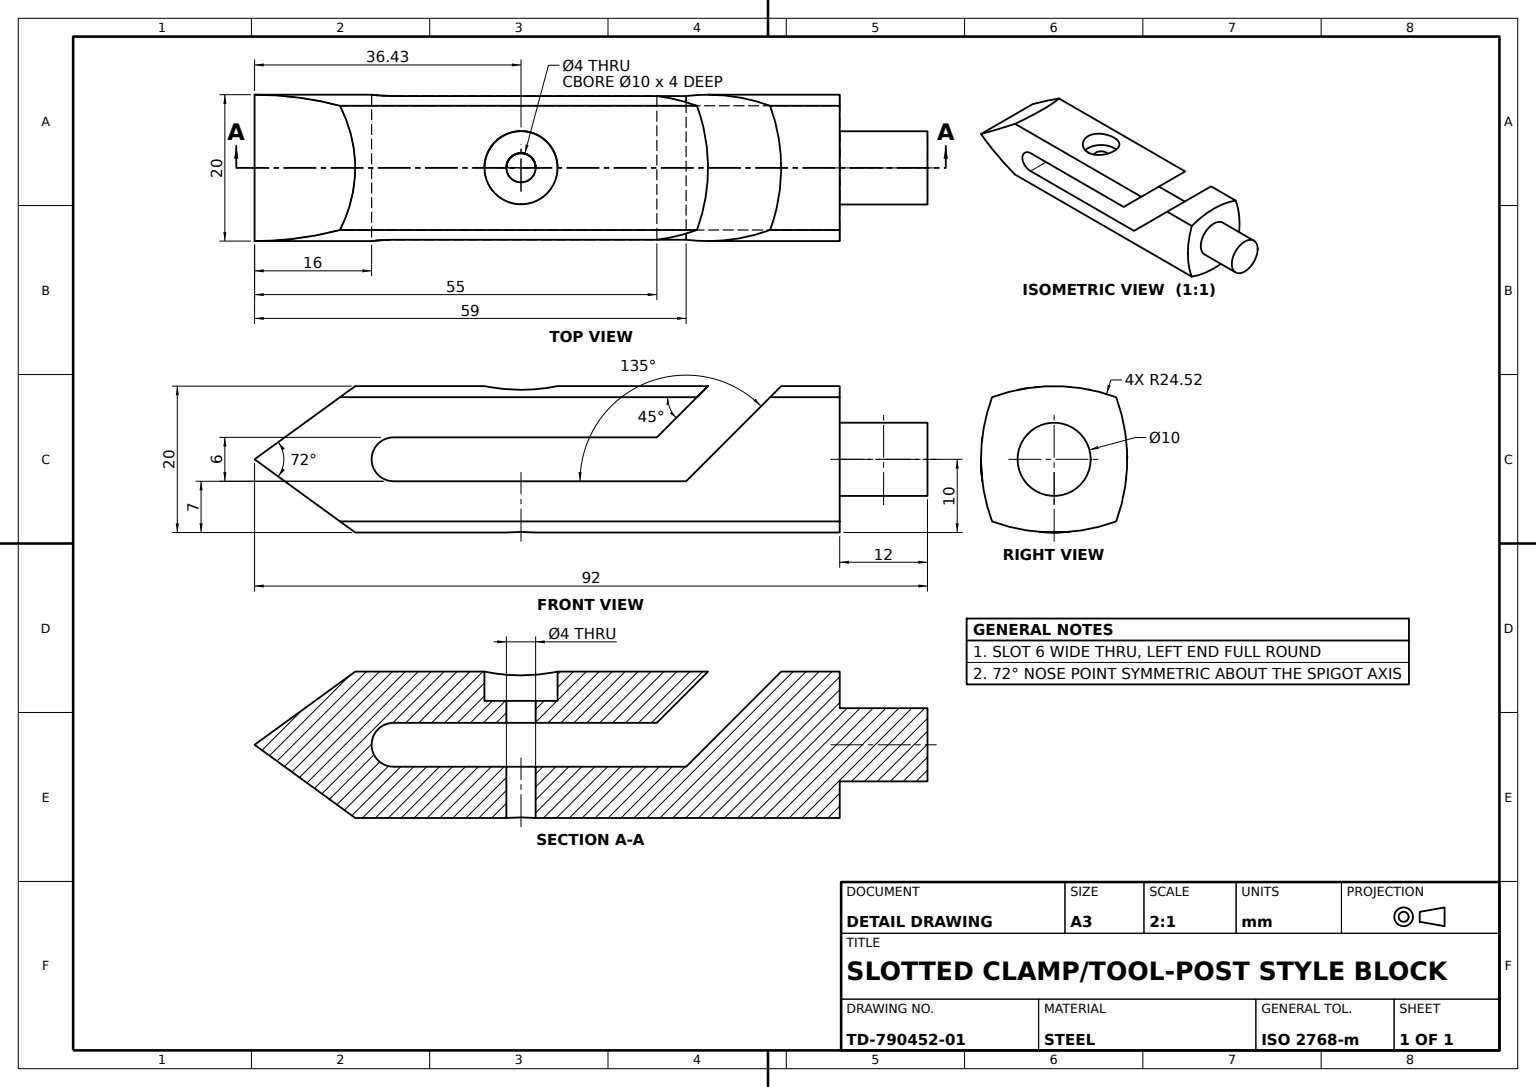
SolidWorks part; units mm, degrees
material "Plain Carbon Steel"
ref_plane "Front Plane" through (0, 0, 0) normal (0, 0, 1) x (1, 0, 0)
ref_plane "Top Plane" through (0, 0, 0) normal (0, 1, 0) x (1, 0, 0)
ref_plane "Right Plane" through (0, 0, 0) normal (1, 0, 0) x (0, 0, -1)
sketch "Pin Body Profile" plane through (0, 0, 0) normal (1, 0, 0) x (0, 0, -1)
  line L0 (0, 0) -> (0, 7.0176) construction
  line L1 (0, 0) -> (-5.821, 0) construction
  line L3 (-8.4853, -8.4853) -> (8.4853, 8.4853) construction
  arc A0 (-8.4853, -8.4853) -> (-8.4853, 8.4853) centre (14.5241, 0) cw
  arc A1 (-8.4853, 8.4853) -> (8.4853, 8.4853) centre (0, -14.5241) cw
  arc A2 (8.4853, -8.4853) -> (8.4853, 8.4853) centre (-14.5241, 0) ccw
  arc A3 (-8.4853, -8.4853) -> (8.4853, -8.4853) centre (0, 14.5241) ccw
  point P6 (-10, 0)
  point P10 (0, 10)
  dimension "D1" = 10
  dimension "D2" = 10
  dimension "D3" = 24
extrude "Pin Body 80mm" add sketch "Pin Body Profile" along normal blind 80
sketch "Arrow Nose Profile 72deg" plane through (0, 0, 0) normal (0, 0, 1) x (1, 0, 0)
  line L0 (0, 0) -> (13.7638, 10)
  line L1 (80, 10) -> (0, 10) construction
  line L2 (0, 0) -> (13.7638, -10)
  line L3 (0, -10) -> (80, -10) construction
  line L4 (0, 0) -> (15.5307, 0) construction
  line L5 (13.7638, 10) -> (0, 10)
  line L6 (0, 10) -> (0, -10)
  line L7 (0, -10) -> (13.7638, -10)
  dimension "D1" = 72
extrude "Arrow Nose Cut" cut sketch "Arrow Nose Profile 72deg" against normal through all both and the other way through all contours L5 L6 L0 | L6 L7 L2
sketch "Slot and Step Profile" plane through (0, 0, 0) normal (0, 0, 1) x (1, 0, 0)
  line L0 (72, 10) -> (59, -3)
  line L1 (80, 10) -> (13.7638, 10) construction
  line L2 (59, -3) -> (19, -3)
  line L3 (19, 3) -> (55, 3)
  line L4 (55, 3) -> (62, 10)
  line L5 (80, -8.4853) -> (80, 8.4853) construction
  line L6 (62, 10) -> (72, 10)
  arc A0 (19, -3) -> (19, 3) centre (19, 0) cw
  dimension "D1" = 8
  dimension "D2" = 19
  dimension "D3" = 135
  dimension "D4" = 6
  dimension "D5" = 10
extrude "Slot and Step Cut" cut sketch "Slot and Step Profile" against normal through all both and the other way through all
sketch "Spigot Profile Ø10" plane through (80, 0, 0) normal (1, 0, 0) x (0, 0, -1)
  circle A0 centre (0, 0) radius 5
  dimension "D1" = 10
extrude "Spigot Ø10x12" add sketch "Spigot Profile Ø10" along normal blind 12
hole_wizard "Counterbored Hole Ø4" positions "3DSketch1" profile "Sketch6" legacy
sketch3d "3DSketch1"
  line L1 (80, 10, -0.0307) -> (25.602, 10, -0.0307) construction
  arc A0 (80, 8.4853, -8.4853) -> (80, 8.4853, 8.4853) centre (80, -14.5241, 0) ccw construction
  point P0 (36.4275, 10, -0.0307)
  point P6 (104.5241, -14.5241, 0)
  dimension "D1" = 50
sketch "Sketch6" plane through (36.4275, 10, -0.0307) normal (1, 0, 0) x (0, 0.0013, 1)
  line L0 (0, 0) -> (0, 100)
  line L1 (0, 100) -> (2, 100)
  line L2 (2, 100) -> (2, 4)
  line L3 (2, 4) -> (5, 4)
  line L4 (5, 4) -> (5, 0)
  line L5 (5, 0) -> (0, 0)
  line L6 (0, 110) -> (0, -10) construction
  dimension "Diameter" = 4
  dimension "Depth" = 100
  dimension "C-Bore Diameter" = 10
  dimension "C-Bore Depth" = 4
